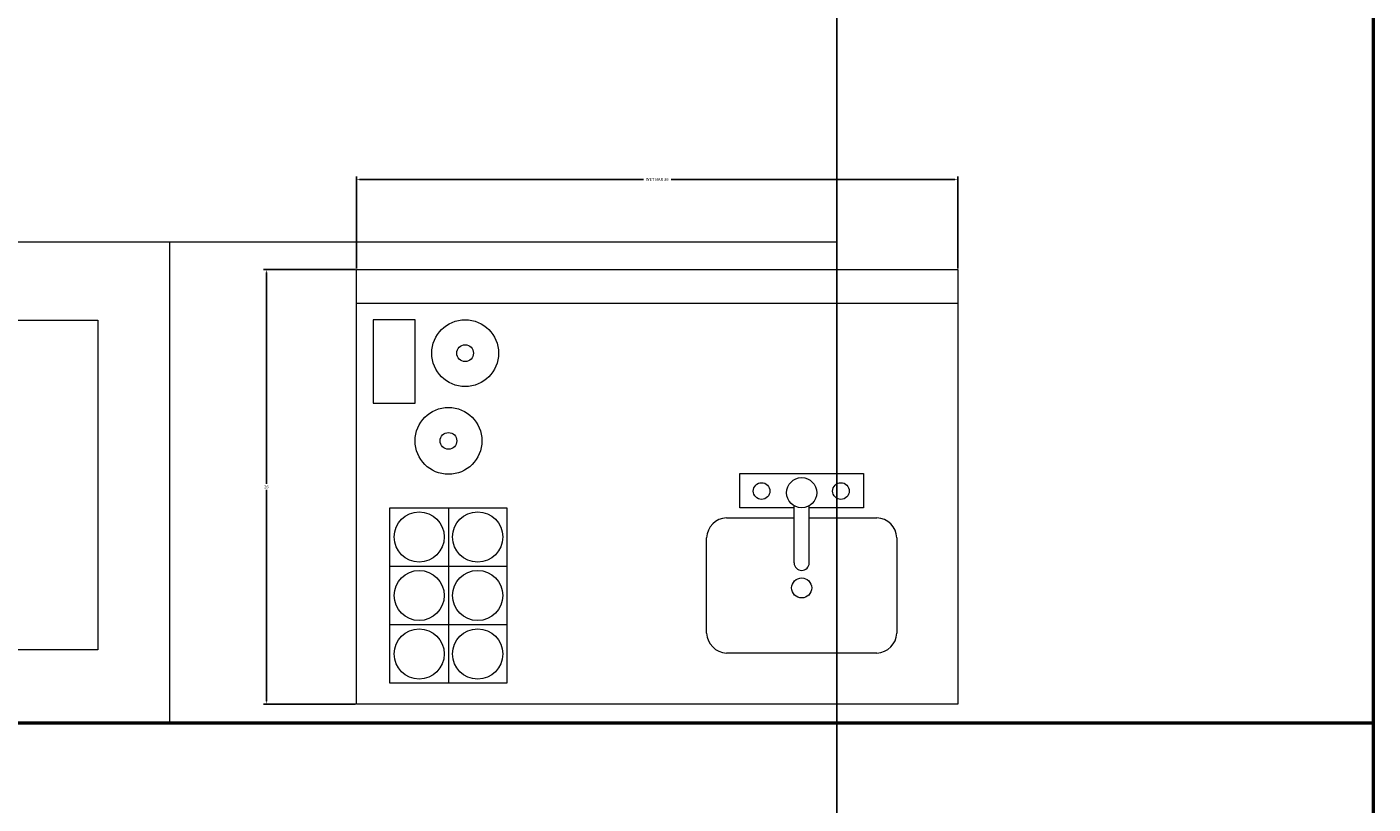
# Model space of a CAD drawing. Units: inches. Extents: x 5375 to 6084, y 16106 to 17259.
# Tile 28 of 32: x 5866 to 5946, y 16776 to 16822. Entities that reach past the tile are written whole.
import ezdxf

# ---------------------------------------------------------------- set-up
doc = ezdxf.new("R2010")
doc.units = ezdxf.units.IN
for name, color, linetype, lineweight in [('A-ANNO-DIMS', 2, 'Continuous', 18), ('A-FLOR-CASE', 3, 'Continuous', 18), ('A-FLOR-FIXT', 3, 'Continuous', 18), ('WALL', 6, 'Continuous', 50)]:
    doc.layers.add(name, color=color, linetype=linetype, lineweight=lineweight)
doc.styles.get("Standard").update_dxf_attribs({"font": 'arial.ttf'})
doc.dimstyles.get("Standard").update_dxf_attribs({"dimtxt": 0.18, "dimasz": 0.18, "dimexe": 0.18, "dimexo": 0.0625, "dimgap": 0.09, "dimtad": 0, "dimtih": 1, "dimtoh": 1, "dimdec": 4, "dimzin": 0, "dimdsep": 46, "dimtxsty": 'Standard', "dimcen": 0.09, "dimadec": 0, "dimazin": 0, "dimtfac": 1, "dimtdec": 4, "dimtofl": 0, "dimtmove": 0, "dimatfit": 3, "dimfxl": 1, "dimtolj": 1, "dimtzin": 0, "dimarcsym": 0})

# ---------------------------------------------------------------- blocks, each defined once
blk = doc.blocks.new('Wet Bar')
for p, q in [((0, 0), (36, 0)), ((0, -26), (0, 0)), ((36, 0), (36, -26)), ((0, -2), (36, -2)), ((3.5, -3), (1, -3)), ((1, -3), (1, -8)), ((3.5, -8), (3.5, -3)), ((1, -8), (3.5, -8)), ((2, -14.25), (9, -14.25)), ((2, -24.75), (2, -14.25)), ((5.5, -14.25), (5.5, -24.75)), ((9, -14.25), (9, -24.75)), ((26.2, -17.55), (26.2, -14.1284)), ((27.1001, -17.55), (27.1001, -14.1284)), ((2, -17.75), (9, -17.75)), ((9, -21.25), (2, -21.25)), ((9, -24.75), (2, -24.75)), ((36, -26), (0, -26))]:
    blk.add_line(p, q)
for points in [[(26.2, -14.25), (22.95, -14.25), (22.95, -12.2), (26.75, -12.2)], [(26.7487, -12.2), (30.3501, -12.2), (30.3501, -14.25), (27.1001, -14.25)], [(22.15, -14.85), (26.2, -14.85)], [(27.1001, -14.85), (31.15, -14.85)], [(20.95, -21.75), (20.95, -16.05)], [(32.3501, -16.05), (32.3501, -21.75)], [(31.15, -22.95), (22.15, -22.95)]]:
    blk.add_lwpolyline(points)
for centre, radius in [((6.5, -5), 2), ((6.5, -5), 0.5), ((5.5, -10.25), 2), ((5.5, -10.25), 0.5), ((24.25, -13.25), 0.5), ((26.65, -13.35), 0.9), ((29, -13.25), 0.5), ((3.75, -16), 1.5), ((7.25, -16), 1.5), ((3.75, -19.5), 1.5), ((7.25, -19.5), 1.5), ((26.65, -19.05), 0.6), ((3.75, -23), 1.5), ((7.25, -23), 1.5)]:
    blk.add_circle(centre, radius)
for centre, radius, start, end in [((22.2251, -16.125), 1.2772, 93.36646, 176.6335), ((31.075, -16.125), 1.2772, 3.366461, 86.63354), ((26.65, -17.55), 0.45, 180, 0), ((22.2251, -21.675), 1.2772, 183.3665, 266.6335), ((31.075, -21.675), 1.2772, 273.3665, 356.6335)]:
    blk.add_arc(centre, radius, start, end)
blk = doc.blocks.new('*D28')
at = {"layer": 'A-ANNO-DIMS', "color": 0, "lineweight": -2, "transparency": 16777216}
for p, q in [((5885.258, 16807.764), (5885.258, 16813.282)), ((5921.258, 16807.764), (5921.258, 16813.282)), ((5885.438, 16813.102), (5902.428, 16813.102)), ((5921.078, 16813.102), (5904.089, 16813.102))]:
    blk.add_line(p, q, dxfattribs=at)
at = {"layer": 'A-ANNO-DIMS', "color": 0, "transparency": 16777216}
for points in [[(5885.438, 16813.132), (5885.438, 16813.072), (5885.258, 16813.102)], [(5921.078, 16813.132), (5921.078, 16813.072), (5921.258, 16813.102)]]:
    blk.add_solid(points, dxfattribs=at)
at = {"layer": 'Defpoints', "color": 0, "transparency": 16777216}
for p in [(5921.258, 16813.102), (5885.258, 16807.702), (5921.258, 16807.702)]:
    blk.add_point(p, dxfattribs=at)
at = {"layer": 'A-ANNO-DIMS', "color": 0, "transparency": 16777216, "insert": (5903.258, 16813.102), "char_height": 0.18, "attachment_point": 5}
blk.add_mtext('\\A1;WET BAR 36', dxfattribs=at)
blk = doc.blocks.new('*D29')
at = {"layer": 'A-ANNO-DIMS', "color": 0, "lineweight": -2, "transparency": 16777216}
for p, q in [((5885.196, 16807.702), (5879.678, 16807.702)), ((5879.858, 16807.522), (5879.858, 16794.884)), ((5879.858, 16781.882), (5879.858, 16794.52)), ((5885.196, 16781.702), (5879.678, 16781.702))]:
    blk.add_line(p, q, dxfattribs=at)
at = {"layer": 'A-ANNO-DIMS', "color": 0, "transparency": 16777216}
for points in [[(5879.828, 16807.522), (5879.888, 16807.522), (5879.858, 16807.702)], [(5879.828, 16781.882), (5879.888, 16781.882), (5879.858, 16781.702)]]:
    blk.add_solid(points, dxfattribs=at)
at = {"layer": 'Defpoints', "color": 0, "transparency": 16777216}
for p in [(5879.858, 16807.702), (5885.258, 16807.702), (5885.258, 16781.702)]:
    blk.add_point(p, dxfattribs=at)
at = {"layer": 'A-ANNO-DIMS', "color": 0, "transparency": 16777216, "insert": (5879.858, 16794.702), "char_height": 0.18, "attachment_point": 5}
blk.add_mtext('\\A1;26', dxfattribs=at)
blk = doc.blocks.new('*D44')
at = {"layer": 'A-ANNO-DIMS', "color": 0, "lineweight": -2, "transparency": 16777216}
for p, q in [((5914.003, 16886.533), (5914.003, 16106.483)), ((5946.12, 16886.533), (5946.12, 16106.483)), ((5914.183, 16106.663), (5929.598, 16106.663)), ((5945.94, 16106.663), (5930.525, 16106.663))]:
    blk.add_line(p, q, dxfattribs=at)
at = {"layer": 'A-ANNO-DIMS', "color": 0, "transparency": 16777216}
for points in [[(5914.183, 16106.693), (5914.183, 16106.633), (5914.003, 16106.663)], [(5945.94, 16106.693), (5945.94, 16106.633), (5946.12, 16106.663)]]:
    blk.add_solid(points, dxfattribs=at)
at = {"layer": 'Defpoints', "color": 0, "transparency": 16777216}
for p in [(5914.003, 16886.596), (5946.12, 16886.596), (5914.003, 16106.663)]:
    blk.add_point(p, dxfattribs=at)
at = {"layer": 'A-ANNO-DIMS', "color": 0, "transparency": 16777216, "insert": (5930.062, 16106.663), "char_height": 0.18, "attachment_point": 5}
blk.add_mtext('\\A1;32.117', dxfattribs=at)

msp = doc.modelspace()

# ---------------------------------------------------------------- linework, layer by layer
at = {"layer": 'A-FLOR-CASE'}
for p, q in [((5914.0033, 16809.3651), (5914.0033, 16886.5956)), ((5826.1199, 16809.3651), (5914.0033, 16809.3651)), ((5874.0547, 16809.3651), (5874.0547, 16780.5793))]:
    msp.add_line(p, q, dxfattribs=at)
at = {"layer": 'A-FLOR-FIXT'}
msp.add_lwpolyline([(5869.7591, 16784.9398), (5832.8693, 16784.9398), (5832.8693, 16804.67), (5869.7591, 16804.67)], close=True, dxfattribs=at)
at = {"layer": 'WALL'}
for p, q in [((5946.1199, 16891.5793), (5946.1199, 16771.5793)), ((5826.1199, 16780.5793), (5946.1199, 16780.5793))]:
    msp.add_line(p, q, dxfattribs=at)

# ---------------------------------------------------------------- block references
at = {"layer": 'A-FLOR-FIXT'}
msp.add_blockref('Wet Bar', (5885.2584, 16807.7018), dxfattribs=at)

# ---------------------------------------------------------------- dimensions: what is measured, and where the dimension line sits
at = {"layer": 'A-ANNO-DIMS'}
dim = msp.add_linear_dim(base=(5914.0033, 16106.6631), p1=(5946.1199, 16886.5956), p2=(5914.0033, 16886.5956), dimstyle='Standard', override={"dimdec": 3, "dimlfac": 1, "dimrnd": 0, "dimzin": 0, "dimdsep": 46, "dimlunit": 2}, dxfattribs=at)
dim.commit()
dim.dimension.update_dxf_attribs({"geometry": '*D44', "text_midpoint": (5930.0616, 16106.6631)})
dim = msp.add_linear_dim(base=(5921.2584, 16813.1018), p1=(5885.2584, 16807.7018), p2=(5921.2584, 16807.7018), text='WET BAR <>', dimstyle='Standard', override={"dimdec": 0, "dimlfac": 1, "dimrnd": 0, "dimzin": 0, "dimdsep": 46, "dimlunit": 2}, dxfattribs=at)
dim.commit()
dim.dimension.update_dxf_attribs({"geometry": '*D28', "text_midpoint": (5903.2584, 16813.1018)})
dim = msp.add_linear_dim(base=(5879.8584, 16807.7018), p1=(5885.2584, 16781.7018), p2=(5885.2584, 16807.7018), angle=90, dimstyle='Standard', override={"dimdec": 0, "dimlfac": 1, "dimrnd": 0, "dimzin": 0, "dimdsep": 46, "dimlunit": 2}, dxfattribs=at)
dim.commit()
dim.dimension.update_dxf_attribs({"geometry": '*D29', "text_midpoint": (5879.8584, 16794.7018)})

doc.saveas('drawing.dxf')
